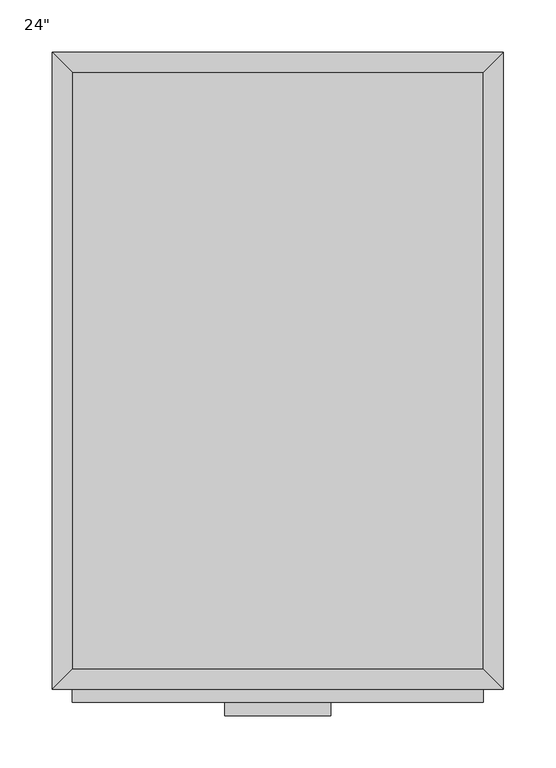
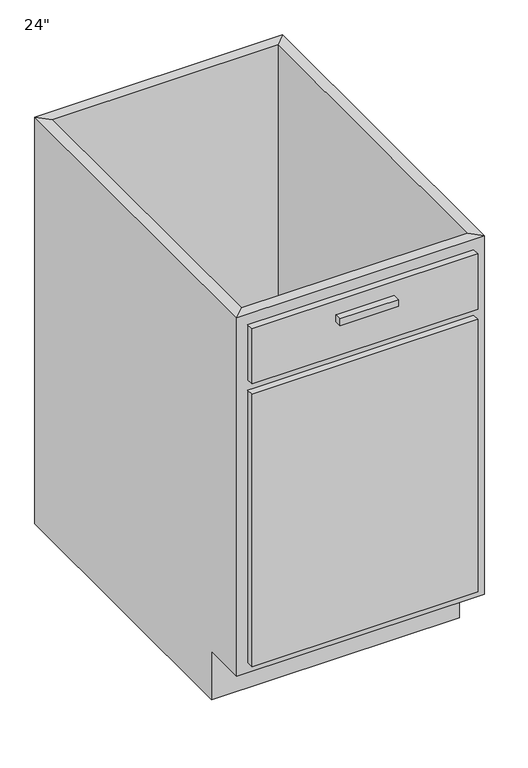
"""IFC4 building model written with IfcOpenShell, lengths in millimetres: furniture geometry."""

from ifc_helpers import new_model, si_unit, frame, origin, place, context, project, spatial, polyline, outline, extrude, faceted_brep, source, transform, mapped, element, save


def furniture_39db8c53(model_context):
    return source(origin(), model_context, "Body", "SolidModel", [
        faceted_brep([(215.5877049, -590.55, 749.3), (215.5877049, -590.55, 88.9), (-178.1122951, -590.55, 88.9), (-178.1122951, -590.55, 749.3), (-197.1622951, -609.6, 749.3), (234.6377049, -609.6, 749.3), (-197.1622951, -609.6, 88.9), (234.6377049, -609.6, 88.9), (-178.1122951, -533.4, 88.9), (-178.1122951, -19.05, 88.9), (-178.1122951, -19.05, 749.3), (-197.1622951, 0.0, 749.3), (-197.1622951, 0.0, 0.0), (-197.1622951, -533.4, 0.0), (-197.1622951, -533.4, 88.9), (215.5877049, -19.05, 88.9), (215.5877049, -19.05, 749.3), (234.6377049, 0.0, 749.3), (234.6377049, 0.0, 0.0), (215.5877049, -533.4, 88.9), (234.6377049, -533.4, 88.9), (234.6377049, -533.4, 0.0)], [[[0, 1, 2, 3]], [[0, 3, 4, 5]], [[5, 4, 6, 7]], [[2, 1, 7, 6]], [[3, 2, 8, 9, 10]], [[4, 3, 10, 11]], [[6, 4, 11, 12, 13, 14]], [[2, 6, 14, 8]], [[10, 9, 15, 16]], [[11, 10, 16, 17]], [[12, 11, 17, 18]], [[1, 0, 16, 15, 19]], [[0, 5, 17, 16]], [[5, 7, 20, 21, 18, 17]], [[7, 1, 19, 20]], [[8, 19, 15, 9]], [[18, 21, 13, 12]], [[13, 21, 20, 19, 8, 14]]]),
        extrude(outline(polyline([(215.5877049, -19.05), (215.5877049, -590.55), (-178.1122951, -590.55), (-178.1122951, -19.05), (215.5877049, -19.05)])), frame((0.0, 0.0, 88.9), z_axis=(0.0, 0.0, 1.0), x_axis=(1.0, 0.0, 0.0)), (0.0, 0.0, 1.0), 19.05),
        extrude(outline(polyline([(215.5877049, -622.3), (-178.1122951, -622.3), (-178.1122951, -609.6), (215.5877049, -609.6), (215.5877049, -622.3)])), frame((0.0, 0.0, 628.65), z_axis=(0.0, 0.0, 1.0), x_axis=(1.0, 0.0, 0.0)), (0.0, 0.0, 1.0), 101.6),
        extrude(outline(polyline([(215.5877049, -622.3), (-178.1122951, -622.3), (-178.1122951, -609.6), (215.5877049, -609.6), (215.5877049, -622.3)])), frame((0.0, 0.0, 107.95), z_axis=(0.0, 0.0, 1.0), x_axis=(1.0, 0.0, 0.0)), (0.0, 0.0, 1.0), 501.65),
        extrude(outline(polyline([(69.5377049, -635.0), (-32.0622951, -635.0), (-32.0622951, -622.3), (69.5377049, -622.3), (69.5377049, -635.0)])), frame((0.0, 0.0, 692.15), z_axis=(0.0, 0.0, 1.0), x_axis=(1.0, 0.0, 0.0)), (0.0, 0.0, 1.0), 12.7),
    ])


if __name__ == "__main__":
    model = new_model("IFC4")
    model_context = context("Model", 3, world=origin())
    ifc_project = project(units=[si_unit("LENGTHUNIT", "METRE", prefix="MILLI")], contexts=[model_context])
    site = spatial("IfcSite", under=ifc_project)
    building = spatial("IfcBuilding", under=site)
    placement = place(None, origin())
    furniture_shape = furniture_39db8c53(model_context)
    element("IfcFurniture", 1, ObjectType="24\"", at=placement, inside=building, context=model_context, shape_type="MappedRepresentation", body=[
        mapped(furniture_shape, transform((0.0, 0.0, 0.0), x_axis=(1.0, 0.0, 0.0), y_axis=(0.0, 1.0, 0.0), z_axis=(0.0, 0.0, 1.0))),
    ])
    save(model, "model.ifc")

# Revit data of these elements
# Type "24\""
#   Assembly Code = "C1030410"
#   Depth = 2' - 0"
#   Height = 2' - 5 1/2"
#   Toe Depth = 0' - 3"
#   Toe Height = 0' - 3 1/2"
#   Width = 1' - 5"
#   Cabinet Material = none
#   Door/Drawer Material = none
#   Handle Material = Cabinets - Handles
#   Default Elevation = 0
# Element 1 (IfcFurniture, "24\"")
#   Materials on its faces: "Cabinets", "Cabinets - Handles"
# Materials
#   "Cabinets - Handles": class "Metal", colour RGB 57 57 57, transparency 0
#   "Cabinets": colour RGB 249 249 249, transparency 0
